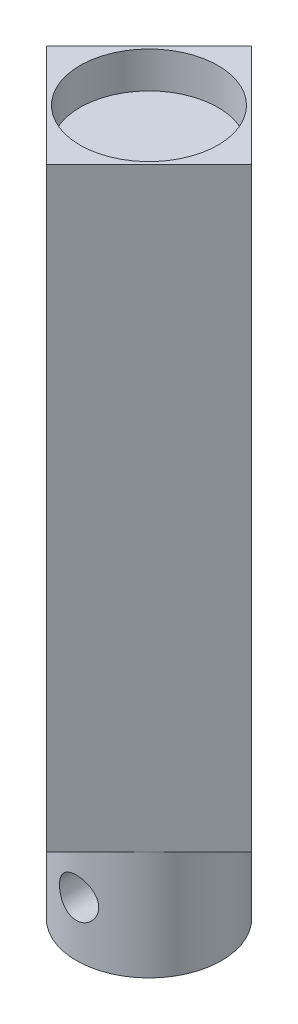
from build123d import *

# Parameters (mm, degrees)
SQUARE_BAR_20X82_DEPTH          = 82
TOP_POCKET_PROFILE_19_R         = 9.5
TOP_POCKET_19X5_DEPTH           = 5
END_SPIGOT_PROFILE_20_R         = 10
END_SPIGOT_20X15_DEPTH          = 15
SKETCH3_3_R                     = 6
SPIGOT_CONTOUR_TRIM_CUT_DEPTH   = 85.403791384
CROSS_TAPPED_HOLE_1_4_28_REACH  = 95.771
CROSS_TAPPED_HOLE_1_4_28_BORE_R = 2.7051


with BuildPart() as part:
    # Square Bar Profile 20 → Square Bar 20x82 (new body)
    with BuildSketch(Plane(origin=(0, 0, 0), x_dir=(1, 0, 0), z_dir=(0, 1, 0))):
        Polygon((-14.142135624, 0), (0, 14.142135624), (14.142135624, 0), (0, -14.142135624), align=None)
    extrude(amount=SQUARE_BAR_20X82_DEPTH)

    # Top Pocket Profile _19 → Top Pocket _19x5 (cut)
    with BuildSketch(Plane(origin=(0, 82, 0), x_dir=(1, 0, 0), z_dir=(0, 1, 0))):
        with Locations(Location((0, 0, 0), (0, 0, 270))):
            Circle(TOP_POCKET_PROFILE_19_R)
    extrude(amount=-TOP_POCKET_19X5_DEPTH, mode=Mode.SUBTRACT)

    # End Spigot Profile _20 → End Spigot _20x15 (add)
    with BuildSketch(Plane.XZ):
        with Locations(Location((0, 0, 0), (0, 0, 45))):
            Circle(END_SPIGOT_PROFILE_20_R)
    extrude(amount=END_SPIGOT_20X15_DEPTH)

    # Sketch3_3 → Spigot Contour Trim Cut (cut, through all)
    with BuildSketch(Plane.XZ):
        with Locations(Location((0, 0, 0), (0, 0, 270))):
            Circle(SKETCH3_3_R)
    extrude(amount=SPIGOT_CONTOUR_TRIM_CUT_DEPTH, mode=Mode.SUBTRACT)

    # Cross Tapped Hole 1-4-28 bore (on position points) → Cross Tapped Hole 1-4-28 (cut, up to next)
    with BuildSketch(Plane(origin=(0, -7.5, 10), x_dir=(1, 0, 0), z_dir=(0, 0, 1)), mode=Mode.PRIVATE) as cross_tapped_hole_1_4_28_sk1:
        Circle(CROSS_TAPPED_HOLE_1_4_28_BORE_R)
    cross_tapped_hole_1_4_28_tool1 = extrude(cross_tapped_hole_1_4_28_sk1.sketch, amount=-CROSS_TAPPED_HOLE_1_4_28_REACH, mode=Mode.PRIVATE) & part.part
    add(cross_tapped_hole_1_4_28_tool1.solids().sort_by_distance((0, -7.5, 10))[0], mode=Mode.SUBTRACT)


solid = part.part
